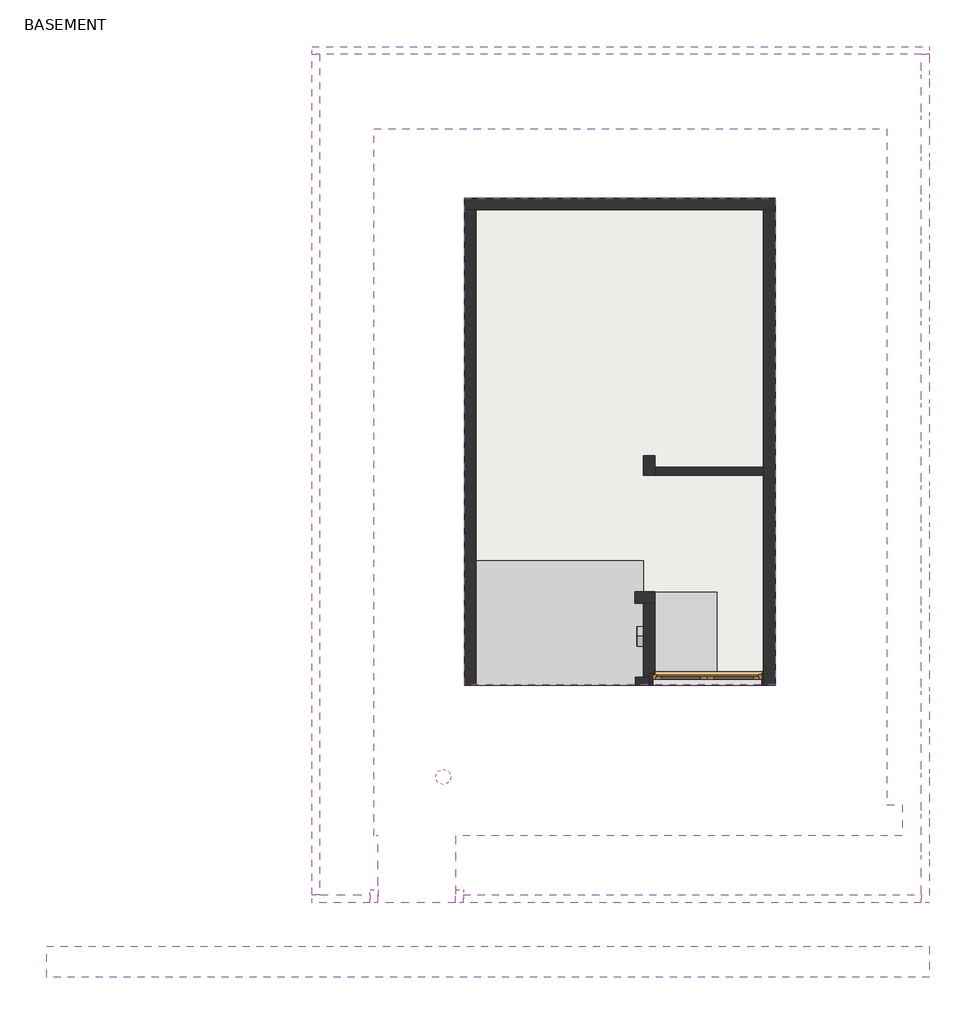
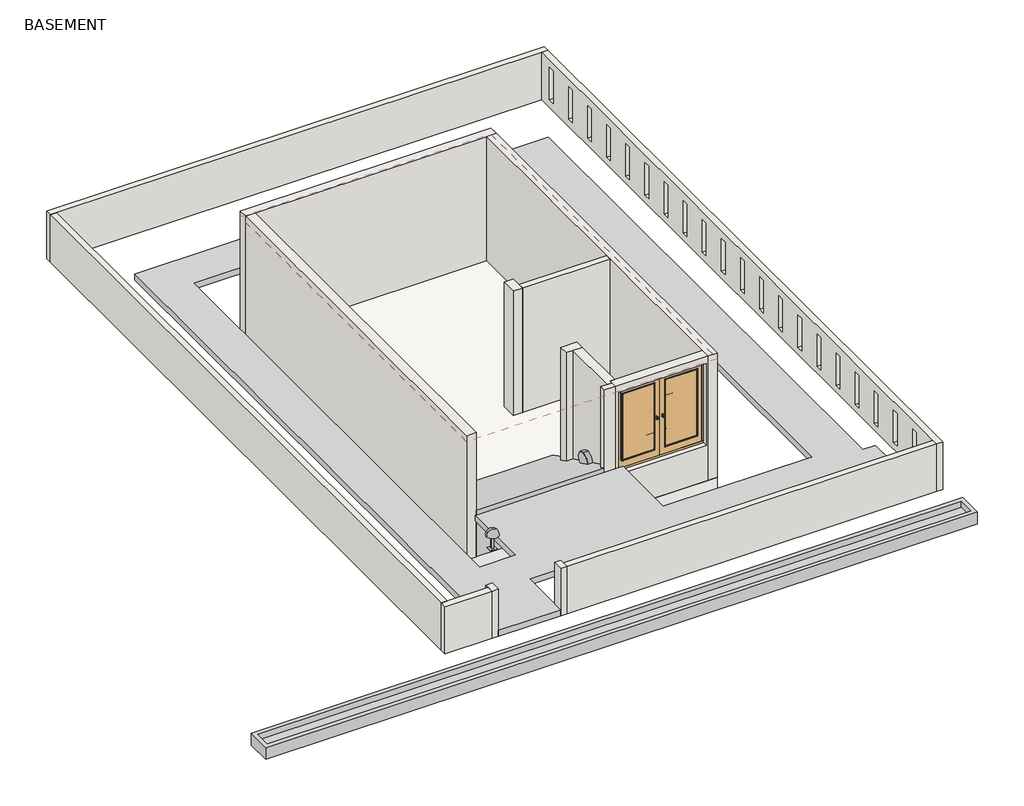
# One storey: 16 walls, 3 proxies, 2 light fixtures, 1 covering, 1 door, 1 slab.
"""IFC4 building model written with IfcOpenShell, lengths in millimetres."""

from ifc_helpers import new_model, si_unit, frame, origin, place, context, project, spatial, polyline, outline, extrude, faceted_brep, transform, mapped, element, save
from components import roads_a759df18, roads_ea5b5616, generic_models_1_generic_models_1_986dd2cf, extdbl_7_2134_x_2110mm_9b31339b, m_sconce_light_flat_round_60w_120v_dc625014, m_table_lamp_hemispheric_60w_120v_fef6e77c

model = new_model("IFC4")

# Units and contexts
model_context = context("Model", 3, world=origin())
ifc_project = project(units=[si_unit("LENGTHUNIT", "METRE", prefix="MILLI")], contexts=[model_context])

# Site, building, storey
site = spatial("IfcSite", under=ifc_project)
building = spatial("IfcBuilding", under=site)
storey = spatial("IfcBuildingStorey", under=building, Name="BASEMENT", Elevation=-3200.4)

# Proxies
placement = place(None, origin())
roads_shape = roads_a759df18(model_context)
element("IfcBuildingElementProxy", 1, Name="Roads", at=placement, inside=storey, context=model_context, shape_type="MappedRepresentation", body=[
    mapped(roads_shape, transform((0.0, 0.0, 0.0), x_axis=(1.0, 0.0, 0.0), y_axis=(0.0, 1.0, 0.0), z_axis=(0.0, 0.0, 1.0))),
])
roads_2_shape = roads_ea5b5616(model_context)
element("IfcBuildingElementProxy", 2, Name="Roads", at=placement, inside=storey, context=model_context, shape_type="MappedRepresentation", body=[
    mapped(roads_2_shape, transform((0.0, 0.0, 0.0), x_axis=(1.0, 0.0, 0.0), y_axis=(0.0, 1.0, 0.0), z_axis=(0.0, 0.0, 1.0))),
])
generic_models_1_generic_models_1_shape = generic_models_1_generic_models_1_986dd2cf(model_context)
element("IfcBuildingElementProxy", 3, Name="Generic Models 1 : Generic Models 1", ObjectType="Generic Models 1 : Generic Models 1", at=placement, inside=storey, context=model_context, shape_type="MappedRepresentation", body=[
    mapped(generic_models_1_generic_models_1_shape, transform((0.0, 0.0, 0.0), x_axis=(1.0, 0.0, 0.0), y_axis=(0.0, 1.0, 0.0), z_axis=(0.0, 0.0, 1.0))),
])

# Covering
element("IfcCovering", 4, ObjectType="2' x 4' ACT System", at=placement, inside=storey, context=model_context, shape_type="SweptSolid", body=[
    extrude(outline(polyline([(-23785.8963079, 6326.0742053), (-17689.8963079, 6326.0742053), (-17689.8963079, -3224.3257947), (-23785.8963079, -3224.3257947), (-23785.8963079, 6326.0742053)])), frame((0.0, 0.0, -152.4), z_axis=(0.0, 0.0, 1.0), x_axis=(1.0, 0.0, 0.0)), (0.0, 0.0, 1.0), 57.15),
])

# Door
extdbl_7_2134_x_2110mm_shape = extdbl_7_2134_x_2110mm_9b31339b(model_context)
element("IfcDoor", 5, ObjectType="ExtDbl (7) : 2134 x 2110mm", at=placement, inside=storey, context=model_context, shape_type="MappedRepresentation", body=[
    mapped(extdbl_7_2134_x_2110mm_shape, transform((-19022.2463079, -3110.0257947, -2286.0), x_axis=(1.0, 0.0, 0.0), y_axis=(0.0, 1.0, 0.0), z_axis=(0.0, 0.0, 1.0))),
])

# Light fixtures
m_sconce_light_flat_round_60w_120v_shape = m_sconce_light_flat_round_60w_120v_dc625014(model_context)
element("IfcLightFixture", 6, ObjectType="M_Sconce Light - Flat Round : 60W - 120V", at=placement, inside=storey, context=model_context, shape_type="MappedRepresentation", body=[
    mapped(m_sconce_light_flat_round_60w_120v_shape, transform((-20166.3963079, -2271.8257947, -4291.8211155), x_axis=(0.0, 1.0, 0.0), y_axis=(-1.0, 0.0, 0.0), z_axis=(0.0, 0.0, 1.0))),
])
m_table_lamp_hemispheric_60w_120v_shape = m_table_lamp_hemispheric_60w_120v_fef6e77c(model_context)
element("IfcLightFixture", 7, ObjectType="M_Table Lamp - Hemispheric : 60W - 120V", at=placement, inside=storey, context=model_context, shape_type="MappedRepresentation", body=[
    mapped(m_table_lamp_hemispheric_60w_120v_shape, transform((-24204.9963079, -5027.7257947, -1676.4), x_axis=(1.0, 0.0, 0.0), y_axis=(0.0, 1.0, 0.0), z_axis=(0.0, 0.0, 1.0))),
])

# Slab
element("IfcSlab", 8, ObjectType="Generic - 12\"", at=placement, inside=storey, context=model_context, shape_type="SweptSolid", body=[
    extrude(outline(polyline([(-23785.8963079, 6326.0742053), (-17689.8963079, 6326.0742053), (-17689.8963079, -3224.3257947), (-23785.8963079, -3224.3257947), (-23785.8963079, 6326.0742053)])), frame((0.0, 0.0, -3505.2), z_axis=(0.0, 0.0, 1.0), x_axis=(1.0, 0.0, 0.0)), (0.0, 0.0, 1.0), 304.8),
])

# Walls
element("IfcWall", 9, ObjectType="Generic - 6\"", at=placement, inside=storey, context=model_context, shape_type="SweptSolid", body=[
    extrude(outline(polyline([(-20052.0963079, 1042.8742053), (-17918.4963079, 1042.8742053), (-17918.4963079, 890.4742053), (-20052.0963079, 890.4742053), (-20052.0963079, 1042.8742053)])), frame((0.0, 0.0, -3200.4), z_axis=(0.0, 0.0, 1.0), x_axis=(1.0, 0.0, 0.0)), (0.0, 0.0, 1.0), 3200.4),
])
element("IfcWall", 10, ObjectType="Generic - 6\"", at=placement, inside=storey, context=model_context, shape_type="Brep", body=[
    faceted_brep([(-20433.0963079, -3224.3257947, -3200.4), (-20166.3963079, -3224.3257947, -3200.4), (-20166.3963079, -3224.3257947, 0.0), (-20433.0963079, -3224.3257947, 0.0), (-20433.0963079, -3071.9257947, -3200.4), (-20433.0963079, -3071.9257947, 0.0), (-20280.6963079, -3071.9257947, 0.0), (-20166.3963079, -3071.9257947, 0.0), (-20166.3963079, -3071.9257947, -3200.4), (-20280.6963079, -3071.9257947, -3200.4)], [[[0, 1, 2, 3]], [[4, 5, 6, 7, 8, 9]], [[1, 0, 4, 9, 8]], [[2, 1, 8, 7]], [[3, 2, 7, 6, 5]], [[0, 3, 5, 4]]]),
])
element("IfcWall", 11, ObjectType="Generic - 6\"", at=placement, inside=storey, context=model_context, shape_type="Brep", body=[
    faceted_brep([(-26783.0963079, 9145.4742053, -1981.2), (-26630.6963079, 9145.4742053, -1981.2), (-14819.6963079, 9145.4742053, -1981.2), (-14667.2963079, 9145.4742053, -1981.2), (-14667.2963079, 9145.4742053, -762.0), (-14819.6963079, 9145.4742053, -762.0), (-26630.6963079, 9145.4742053, -762.0), (-26783.0963079, 9145.4742053, -762.0), (-26783.0963079, 9297.8742053, -1981.2), (-26783.0963079, 9297.8742053, -762.0), (-14667.2963079, 9297.8742053, -762.0), (-14667.2963079, 9297.8742053, -1981.2)], [[[0, 1, 2, 3, 4, 5, 6, 7]], [[8, 9, 10, 11]], [[3, 2, 1, 0, 8, 11]], [[7, 6, 5, 4, 10, 9]], [[4, 3, 11, 10]], [[0, 7, 9, 8]]]),
])
element("IfcWall", 12, ObjectType="Generic - 6\"", at=placement, inside=storey, context=model_context, shape_type="Brep", body=[
    faceted_brep([(-14819.6963079, 9145.4742053, -1981.2), (-14819.6963079, -7339.1257947, -1981.2), (-14819.6963079, -7491.5257947, -1981.2), (-14819.6963079, -7491.5257947, -762.0), (-14819.6963079, -7339.1257947, -762.0), (-14819.6963079, 9145.4742053, -762.0), (-14819.6963079, -6490.3219748, -982.1857398), (-14819.6963079, -6642.4176399, -982.1857398), (-14819.6963079, -6642.4176399, -1818.7118977), (-14819.6963079, -6490.3219748, -1818.7118977), (-14819.6963079, 8667.8340702, -1794.1092134), (-14819.6963079, 8819.9297353, -1794.1092134), (-14819.6963079, 8819.9297353, -957.5830554), (-14819.6963079, 8667.8340702, -957.5830554), (-14819.6963079, 8014.1270137, -1795.4040915), (-14819.6963079, 8014.1270137, -958.8779336), (-14819.6963079, 7862.0313486, -958.8779336), (-14819.6963079, 7862.0313486, -1795.4040915), (-14819.6963079, 7208.3242921, -1796.6989696), (-14819.6963079, 7208.3242921, -960.1728117), (-14819.6963079, 7056.228627, -960.1728117), (-14819.6963079, 7056.228627, -1796.6989696), (-14819.6963079, 6402.5215705, -1797.9938477), (-14819.6963079, 6402.5215705, -961.4676898), (-14819.6963079, 6250.4259054, -961.4676898), (-14819.6963079, 6250.4259054, -1797.9938477), (-14819.6963079, 5596.7188489, -1799.2887259), (-14819.6963079, 5596.7188489, -962.7625679), (-14819.6963079, 5444.6231838, -962.7625679), (-14819.6963079, 5444.6231838, -1799.2887259), (-14819.6963079, 4790.9161273, -1800.583604), (-14819.6963079, 4790.9161273, -964.057446), (-14819.6963079, 4638.8204623, -964.057446), (-14819.6963079, 4638.8204623, -1800.583604), (-14819.6963079, 3985.1134058, -1801.8784821), (-14819.6963079, 3985.1134058, -965.3523242), (-14819.6963079, 3833.0177407, -965.3523242), (-14819.6963079, 3833.0177407, -1801.8784821), (-14819.6963079, 3179.3106842, -1803.1733602), (-14819.6963079, 3179.3106842, -966.6472023), (-14819.6963079, 3027.2150191, -966.6472023), (-14819.6963079, 3027.2150191, -1803.1733602), (-14819.6963079, 2373.5079626, -1804.4682384), (-14819.6963079, 2373.5079626, -967.9420804), (-14819.6963079, 2221.4122975, -967.9420804), (-14819.6963079, 2221.4122975, -1804.4682384), (-14819.6963079, 1567.705241, -1805.7631165), (-14819.6963079, 1567.705241, -969.2369585), (-14819.6963079, 1415.6095759, -969.2369585), (-14819.6963079, 1415.6095759, -1805.7631165), (-14819.6963079, 761.9025194, -1807.0579946), (-14819.6963079, 761.9025194, -970.5318367), (-14819.6963079, 609.8068543, -970.5318367), (-14819.6963079, 609.8068543, -1807.0579946), (-14819.6963079, -43.9002022, -1808.3528727), (-14819.6963079, -43.9002022, -971.8267148), (-14819.6963079, -195.9958672, -971.8267148), (-14819.6963079, -195.9958672, -1808.3528727), (-14819.6963079, -849.7029238, -1809.6477508), (-14819.6963079, -849.7029238, -973.1215929), (-14819.6963079, -1001.7985888, -973.1215929), (-14819.6963079, -1001.7985888, -1809.6477508), (-14819.6963079, -1655.5056453, -1810.942629), (-14819.6963079, -1655.5056453, -974.416471), (-14819.6963079, -1807.6013104, -974.416471), (-14819.6963079, -1807.6013104, -1810.942629), (-14819.6963079, -2461.3083669, -1812.2375071), (-14819.6963079, -2461.3083669, -975.7113492), (-14819.6963079, -2613.404032, -975.7113492), (-14819.6963079, -2613.404032, -1812.2375071), (-14819.6963079, -3267.1110885, -1813.5323852), (-14819.6963079, -3267.1110885, -977.0062273), (-14819.6963079, -3419.2067536, -977.0062273), (-14819.6963079, -3419.2067536, -1813.5323852), (-14819.6963079, -4072.9138101, -1814.8272633), (-14819.6963079, -4072.9138101, -978.3011054), (-14819.6963079, -4225.0094752, -978.3011054), (-14819.6963079, -4225.0094752, -1814.8272633), (-14819.6963079, -4878.7165317, -1816.1221415), (-14819.6963079, -4878.7165317, -979.5959835), (-14819.6963079, -5030.8121968, -979.5959835), (-14819.6963079, -5030.8121968, -1816.1221415), (-14819.6963079, -5684.5192533, -980.8908616), (-14819.6963079, -5836.6149183, -980.8908616), (-14819.6963079, -5836.6149183, -1817.4170196), (-14819.6963079, -5684.5192533, -1817.4170196), (-14667.2963079, -7491.5257947, -1981.2), (-14667.2963079, 9145.4742053, -1981.2), (-14667.2963079, 9145.4742053, -762.0), (-14667.2963079, -7491.5257947, -762.0), (-14667.2963079, -6642.4176399, -982.1857398), (-14667.2963079, -6490.3219748, -982.1857398), (-14667.2963079, -6490.3219748, -1818.7118977), (-14667.2963079, -6642.4176399, -1818.7118977), (-14667.2963079, 8819.9297353, -1794.1092134), (-14667.2963079, 8667.8340702, -1794.1092134), (-14667.2963079, 8667.8340702, -957.5830554), (-14667.2963079, 8819.9297353, -957.5830554), (-14667.2963079, 8014.1270137, -958.8779336), (-14667.2963079, 8014.1270137, -1795.4040915), (-14667.2963079, 7862.0313486, -1795.4040915), (-14667.2963079, 7862.0313486, -958.8779336), (-14667.2963079, 7208.3242921, -960.1728117), (-14667.2963079, 7208.3242921, -1796.6989696), (-14667.2963079, 7056.228627, -1796.6989696), (-14667.2963079, 7056.228627, -960.1728117), (-14667.2963079, 6402.5215705, -961.4676898), (-14667.2963079, 6402.5215705, -1797.9938477), (-14667.2963079, 6250.4259054, -1797.9938477), (-14667.2963079, 6250.4259054, -961.4676898), (-14667.2963079, 5596.7188489, -962.7625679), (-14667.2963079, 5596.7188489, -1799.2887259), (-14667.2963079, 5444.6231838, -1799.2887259), (-14667.2963079, 5444.6231838, -962.7625679), (-14667.2963079, 4790.9161273, -964.057446), (-14667.2963079, 4790.9161273, -1800.583604), (-14667.2963079, 4638.8204623, -1800.583604), (-14667.2963079, 4638.8204623, -964.057446), (-14667.2963079, 3985.1134058, -965.3523242), (-14667.2963079, 3985.1134058, -1801.8784821), (-14667.2963079, 3833.0177407, -1801.8784821), (-14667.2963079, 3833.0177407, -965.3523242), (-14667.2963079, 3179.3106842, -966.6472023), (-14667.2963079, 3179.3106842, -1803.1733602), (-14667.2963079, 3027.2150191, -1803.1733602), (-14667.2963079, 3027.2150191, -966.6472023), (-14667.2963079, 2373.5079626, -967.9420804), (-14667.2963079, 2373.5079626, -1804.4682384), (-14667.2963079, 2221.4122975, -1804.4682384), (-14667.2963079, 2221.4122975, -967.9420804), (-14667.2963079, 1567.705241, -969.2369585), (-14667.2963079, 1567.705241, -1805.7631165), (-14667.2963079, 1415.6095759, -1805.7631165), (-14667.2963079, 1415.6095759, -969.2369585), (-14667.2963079, 761.9025194, -970.5318367), (-14667.2963079, 761.9025194, -1807.0579946), (-14667.2963079, 609.8068543, -1807.0579946), (-14667.2963079, 609.8068543, -970.5318367), (-14667.2963079, -43.9002022, -971.8267148), (-14667.2963079, -43.9002022, -1808.3528727), (-14667.2963079, -195.9958672, -1808.3528727), (-14667.2963079, -195.9958672, -971.8267148), (-14667.2963079, -849.7029238, -973.1215929), (-14667.2963079, -849.7029238, -1809.6477508), (-14667.2963079, -1001.7985888, -1809.6477508), (-14667.2963079, -1001.7985888, -973.1215929), (-14667.2963079, -1655.5056453, -974.416471), (-14667.2963079, -1655.5056453, -1810.942629), (-14667.2963079, -1807.6013104, -1810.942629), (-14667.2963079, -1807.6013104, -974.416471), (-14667.2963079, -2461.3083669, -975.7113492), (-14667.2963079, -2461.3083669, -1812.2375071), (-14667.2963079, -2613.404032, -1812.2375071), (-14667.2963079, -2613.404032, -975.7113492), (-14667.2963079, -3267.1110885, -977.0062273), (-14667.2963079, -3267.1110885, -1813.5323852), (-14667.2963079, -3419.2067536, -1813.5323852), (-14667.2963079, -3419.2067536, -977.0062273), (-14667.2963079, -4072.9138101, -978.3011054), (-14667.2963079, -4072.9138101, -1814.8272633), (-14667.2963079, -4225.0094752, -1814.8272633), (-14667.2963079, -4225.0094752, -978.3011054), (-14667.2963079, -4878.7165317, -979.5959835), (-14667.2963079, -4878.7165317, -1816.1221415), (-14667.2963079, -5030.8121968, -1816.1221415), (-14667.2963079, -5030.8121968, -979.5959835), (-14667.2963079, -5836.6149183, -980.8908616), (-14667.2963079, -5684.5192533, -980.8908616), (-14667.2963079, -5684.5192533, -1817.4170196), (-14667.2963079, -5836.6149183, -1817.4170196)], [[[0, 1, 2, 3, 4, 5], [6, 7, 8, 9], [10, 11, 12, 13], [14, 15, 16, 17], [18, 19, 20, 21], [22, 23, 24, 25], [26, 27, 28, 29], [30, 31, 32, 33], [34, 35, 36, 37], [38, 39, 40, 41], [42, 43, 44, 45], [46, 47, 48, 49], [50, 51, 52, 53], [54, 55, 56, 57], [58, 59, 60, 61], [62, 63, 64, 65], [66, 67, 68, 69], [70, 71, 72, 73], [74, 75, 76, 77], [78, 79, 80, 81], [82, 83, 84, 85]], [[86, 87, 88, 89], [90, 91, 92, 93], [94, 95, 96, 97], [98, 99, 100, 101], [102, 103, 104, 105], [106, 107, 108, 109], [110, 111, 112, 113], [114, 115, 116, 117], [118, 119, 120, 121], [122, 123, 124, 125], [126, 127, 128, 129], [130, 131, 132, 133], [134, 135, 136, 137], [138, 139, 140, 141], [142, 143, 144, 145], [146, 147, 148, 149], [150, 151, 152, 153], [154, 155, 156, 157], [158, 159, 160, 161], [162, 163, 164, 165], [166, 167, 168, 169]], [[2, 1, 0, 87, 86]], [[5, 4, 3, 89, 88]], [[0, 5, 88, 87]], [[3, 2, 86, 89]], [[6, 91, 90, 7]], [[8, 93, 92, 9]], [[91, 6, 9, 92]], [[7, 90, 93, 8]], [[12, 97, 96, 13]], [[10, 95, 94, 11]], [[97, 12, 11, 94]], [[13, 96, 95, 10]], [[15, 98, 101, 16]], [[17, 100, 99, 14]], [[98, 15, 14, 99]], [[16, 101, 100, 17]], [[19, 102, 105, 20]], [[21, 104, 103, 18]], [[102, 19, 18, 103]], [[20, 105, 104, 21]], [[23, 106, 109, 24]], [[25, 108, 107, 22]], [[106, 23, 22, 107]], [[24, 109, 108, 25]], [[27, 110, 113, 28]], [[29, 112, 111, 26]], [[110, 27, 26, 111]], [[28, 113, 112, 29]], [[31, 114, 117, 32]], [[33, 116, 115, 30]], [[114, 31, 30, 115]], [[32, 117, 116, 33]], [[35, 118, 121, 36]], [[37, 120, 119, 34]], [[118, 35, 34, 119]], [[36, 121, 120, 37]], [[39, 122, 125, 40]], [[41, 124, 123, 38]], [[122, 39, 38, 123]], [[40, 125, 124, 41]], [[43, 126, 129, 44]], [[45, 128, 127, 42]], [[126, 43, 42, 127]], [[44, 129, 128, 45]], [[47, 130, 133, 48]], [[49, 132, 131, 46]], [[130, 47, 46, 131]], [[48, 133, 132, 49]], [[51, 134, 137, 52]], [[53, 136, 135, 50]], [[134, 51, 50, 135]], [[52, 137, 136, 53]], [[55, 138, 141, 56]], [[57, 140, 139, 54]], [[138, 55, 54, 139]], [[56, 141, 140, 57]], [[59, 142, 145, 60]], [[61, 144, 143, 58]], [[142, 59, 58, 143]], [[60, 145, 144, 61]], [[63, 146, 149, 64]], [[65, 148, 147, 62]], [[146, 63, 62, 147]], [[64, 149, 148, 65]], [[67, 150, 153, 68]], [[69, 152, 151, 66]], [[150, 67, 66, 151]], [[68, 153, 152, 69]], [[71, 154, 157, 72]], [[73, 156, 155, 70]], [[154, 71, 70, 155]], [[72, 157, 156, 73]], [[75, 158, 161, 76]], [[77, 160, 159, 74]], [[158, 75, 74, 159]], [[76, 161, 160, 77]], [[79, 162, 165, 80]], [[81, 164, 163, 78]], [[162, 79, 78, 163]], [[80, 165, 164, 81]], [[82, 167, 166, 83]], [[84, 169, 168, 85]], [[167, 82, 85, 168]], [[83, 166, 169, 84]]]),
])
element("IfcWall", 13, ObjectType="Generic - 6\"", at=placement, inside=storey, context=model_context, shape_type="SweptSolid", body=[
    extrude(outline(polyline([(-23811.2963079, -7339.1257947), (-14819.6963079, -7339.1257947), (-14819.6963079, -7491.5257947), (-23811.2963079, -7491.5257947), (-23811.2963079, -7339.1257947)])), frame((0.0, 0.0, -1981.2), z_axis=(0.0, 0.0, 1.0), x_axis=(1.0, 0.0, 0.0)), (0.0, 0.0, 1.0), 1219.2),
])
element("IfcWall", 14, ObjectType="Generic - 6\"", at=placement, inside=storey, context=model_context, shape_type="SweptSolid", body=[
    extrude(outline(polyline([(-26630.6963079, 9145.4742053), (-26630.6963079, -7339.1257947), (-26783.0963079, -7339.1257947), (-26783.0963079, 9145.4742053), (-26630.6963079, 9145.4742053)])), frame((0.0, 0.0, -1981.2), z_axis=(0.0, 0.0, 1.0), x_axis=(1.0, 0.0, 0.0)), (0.0, 0.0, 1.0), 1219.2),
])
element("IfcWall", 15, ObjectType="Generic - 6\"", at=placement, inside=storey, context=model_context, shape_type="Brep", body=[
    faceted_brep([(-25640.0963079, -7339.1257947, -1981.2), (-26630.6963079, -7339.1257947, -1981.2), (-26783.0963079, -7339.1257947, -1981.2), (-26783.0963079, -7339.1257947, -762.0), (-26630.6963079, -7339.1257947, -762.0), (-25640.0963079, -7339.1257947, -762.0), (-25640.0963079, -7491.5257947, -1981.2), (-25640.0963079, -7491.5257947, -762.0), (-26783.0963079, -7491.5257947, -762.0), (-26783.0963079, -7491.5257947, -1981.2)], [[[0, 1, 2, 3, 4, 5]], [[6, 7, 8, 9]], [[2, 1, 0, 6, 9]], [[5, 4, 3, 8, 7]], [[3, 2, 9, 8]], [[0, 5, 7, 6]]]),
])
element("IfcWall", 16, ObjectType="Generic - 6\"", at=placement, inside=storey, context=model_context, shape_type="Brep", body=[
    faceted_brep([(-25487.6963079, -7491.5257947, -1981.2), (-25487.6963079, -7237.5257947, -1981.2), (-25487.6963079, -7237.5257947, -762.0), (-25487.6963079, -7491.5257947, -762.0), (-25640.0963079, -7491.5257947, -1981.2), (-25640.0963079, -7491.5257947, -762.0), (-25640.0963079, -7339.1257947, -762.0), (-25640.0963079, -7237.5257947, -762.0), (-25640.0963079, -7237.5257947, -1981.2), (-25640.0963079, -7339.1257947, -1981.2)], [[[0, 1, 2, 3]], [[4, 5, 6, 7, 8, 9]], [[1, 0, 4, 9, 8]], [[2, 1, 8, 7]], [[3, 2, 7, 6, 5]], [[0, 3, 5, 4]]]),
])
element("IfcWall", 17, ObjectType="Generic - 6\"", at=placement, inside=storey, context=model_context, shape_type="Brep", body=[
    faceted_brep([(-23811.2963079, -7491.5257947, -1981.2), (-23811.2963079, -7339.1257947, -1981.2), (-23811.2963079, -7237.5257947, -1981.2), (-23811.2963079, -7237.5257947, -762.0), (-23811.2963079, -7339.1257947, -762.0), (-23811.2963079, -7491.5257947, -762.0), (-23963.6963079, -7491.5257947, -1981.2), (-23963.6963079, -7491.5257947, -762.0), (-23963.6963079, -7237.5257947, -762.0), (-23963.6963079, -7237.5257947, -1981.2)], [[[0, 1, 2, 3, 4, 5]], [[6, 7, 8, 9]], [[2, 1, 0, 6, 9]], [[3, 2, 9, 8]], [[5, 4, 3, 8, 7]], [[0, 5, 7, 6]]]),
])
element("IfcWall", 18, ObjectType="Generic - 9\"", at=placement, inside=storey, context=model_context, shape_type="Brep", body=[
    faceted_brep([(-23785.8963079, 6097.4742053, -3200.4), (-23557.2963079, 6097.4742053, -3200.4), (-17918.4963079, 6097.4742053, -3200.4), (-17689.8963079, 6097.4742053, -3200.4), (-17689.8963079, 6097.4742053, 0.0), (-17918.4963079, 6097.4742053, 0.0), (-23557.2963079, 6097.4742053, 0.0), (-23785.8963079, 6097.4742053, 0.0), (-23785.8963079, 6326.0742053, -3200.4), (-23785.8963079, 6326.0742053, 0.0), (-17689.8963079, 6326.0742053, 0.0), (-17689.8963079, 6326.0742053, -3200.4)], [[[0, 1, 2, 3, 4, 5, 6, 7]], [[8, 9, 10, 11]], [[3, 2, 1, 0, 8, 11]], [[7, 6, 5, 4, 10, 9]], [[0, 7, 9, 8]], [[4, 3, 11, 10]]]),
])
element("IfcWall", 19, ObjectType="Generic - 9\"", at=placement, inside=storey, context=model_context, shape_type="SweptSolid", body=[
    extrude(outline(polyline([(-23785.8963079, -3224.3257947), (-23785.8963079, 6097.4742053), (-23557.2963079, 6097.4742053), (-23557.2963079, -3224.3257947), (-23785.8963079, -3224.3257947)])), frame((0.0, 0.0, -3200.4), z_axis=(0.0, 0.0, 1.0), x_axis=(1.0, 0.0, 0.0)), (0.0, 0.0, 1.0), 3200.4),
])
element("IfcWall", 20, ObjectType="Generic - 9\"", at=placement, inside=storey, context=model_context, shape_type="Brep", body=[
    faceted_brep([(-17918.4963079, 6097.4742053, -3200.4), (-17918.4963079, 1042.8742053, -3200.4), (-17918.4963079, 890.4742053, -3200.4), (-17918.4963079, -2995.7257947, -3200.4), (-17918.4963079, -3224.3257947, -3200.4), (-17918.4963079, -3224.3257947, 0.0), (-17918.4963079, -2995.7257947, 0.0), (-17918.4963079, 890.4742053, 0.0), (-17918.4963079, 1042.8742053, 0.0), (-17918.4963079, 6097.4742053, 0.0), (-17689.8963079, 6097.4742053, -3200.4), (-17689.8963079, 6097.4742053, 0.0), (-17689.8963079, -3224.3257947, 0.0), (-17689.8963079, -3224.3257947, -3200.4)], [[[0, 1, 2, 3, 4, 5, 6, 7, 8, 9]], [[10, 11, 12, 13]], [[4, 3, 2, 1, 0, 10, 13]], [[9, 8, 7, 6, 5, 12, 11]], [[0, 9, 11, 10]], [[5, 4, 13, 12]]]),
])
element("IfcWall", 21, ObjectType="Generic - 9\"", at=placement, inside=storey, context=model_context, shape_type="Brep", body=[
    faceted_brep([(-17918.4963079, -2995.7257947, -3200.4), (-20052.0963079, -2995.7257947, -3200.4), (-20166.3963079, -2995.7257947, -3200.4), (-20166.3963079, -2995.7257947, 0.0), (-20052.0963079, -2995.7257947, 0.0), (-17918.4963079, -2995.7257947, 0.0), (-20089.0463079, -2995.7257947, -2286.0), (-17955.4463079, -2995.7257947, -2286.0), (-17955.4463079, -2995.7257947, -176.0), (-20089.0463079, -2995.7257947, -176.0), (-20166.3963079, -3224.3257947, -3200.4), (-17918.4963079, -3224.3257947, -3200.4), (-17918.4963079, -3224.3257947, 0.0), (-20166.3963079, -3224.3257947, 0.0), (-17955.4463079, -3224.3257947, -2286.0), (-20089.0463079, -3224.3257947, -2286.0), (-20089.0463079, -3224.3257947, -176.0), (-17955.4463079, -3224.3257947, -176.0), (-20166.3963079, -3071.9257947, -3200.4), (-20166.3963079, -3071.9257947, 0.0)], [[[0, 1, 2, 3, 4, 5], [6, 7, 8, 9]], [[10, 11, 12, 13], [14, 15, 16, 17]], [[2, 1, 0, 11, 10, 18]], [[3, 2, 18, 10, 13, 19]], [[5, 4, 3, 19, 13, 12]], [[0, 5, 12, 11]], [[6, 15, 14, 7]], [[7, 14, 17, 8]], [[8, 17, 16, 9]], [[15, 6, 9, 16]]]),
])
element("IfcWall", 22, ObjectType="Generic - 9\"", at=placement, inside=storey, context=model_context, shape_type="Brep", body=[
    faceted_brep([(-20280.6963079, 1271.4742053, -3200.4), (-20280.6963079, 890.4742053, -3200.4), (-20280.6963079, 890.4742053, 0.0), (-20280.6963079, 1271.4742053, 0.0), (-20052.0963079, 1271.4742053, -3200.4), (-20052.0963079, 1271.4742053, 0.0), (-20052.0963079, 1042.8742053, 0.0), (-20052.0963079, 890.4742053, 0.0), (-20052.0963079, 890.4742053, -3200.4), (-20052.0963079, 1042.8742053, -3200.4)], [[[0, 1, 2, 3]], [[4, 5, 6, 7, 8, 9]], [[1, 0, 4, 9, 8]], [[3, 2, 7, 6, 5]], [[0, 3, 5, 4]], [[2, 1, 8, 7]]]),
])
element("IfcWall", 23, ObjectType="Generic - 9\"", at=placement, inside=storey, context=model_context, shape_type="Brep", body=[
    faceted_brep([(-20280.6963079, -1624.1257947, -3200.4), (-20280.6963079, -3071.9257947, -3200.4), (-20280.6963079, -3071.9257947, 0.0), (-20280.6963079, -1624.1257947, 0.0), (-20052.0963079, -2995.7257947, -3200.4), (-20052.0963079, -1624.1257947, -3200.4), (-20052.0963079, -1624.1257947, 0.0), (-20052.0963079, -2995.7257947, 0.0), (-20052.0963079, -2995.7257947, -176.0), (-20052.0963079, -2995.7257947, -2286.0), (-20166.3963079, -2995.7257947, -3200.4), (-20166.3963079, -3071.9257947, -3200.4), (-20166.3963079, -3071.9257947, 0.0), (-20166.3963079, -2995.7257947, 0.0)], [[[0, 1, 2, 3]], [[4, 5, 6, 7, 8, 9]], [[1, 0, 5, 4, 10, 11]], [[3, 2, 12, 13, 7, 6]], [[2, 1, 11, 12]], [[11, 10, 13, 12]], [[10, 4, 9, 8, 7, 13]], [[0, 3, 6, 5]]]),
])
element("IfcWall", 24, ObjectType="Generic - 9\"", at=placement, inside=storey, context=model_context, shape_type="Brep", body=[
    faceted_brep([(-20445.7963079, -1624.1257947, -3200.4), (-20280.6963079, -1624.1257947, -3200.4), (-20052.0963079, -1624.1257947, -3200.4), (-20052.0963079, -1624.1257947, 0.0), (-20280.6963079, -1624.1257947, 0.0), (-20445.7963079, -1624.1257947, 0.0), (-20445.7963079, -1395.5257947, -3200.4), (-20445.7963079, -1395.5257947, 0.0), (-20052.0963079, -1395.5257947, 0.0), (-20052.0963079, -1395.5257947, -3200.4)], [[[0, 1, 2, 3, 4, 5]], [[6, 7, 8, 9]], [[2, 1, 0, 6, 9]], [[5, 4, 3, 8, 7]], [[0, 5, 7, 6]], [[3, 2, 9, 8]]]),
])

save(model, "model.ifc")

# Revit data of these elements
# Type "2' x 4' ACT System"
#   Assembly Code = "C3030210"
#   built-in parameter 1002203 = 1 (stored number, unit not read)
#   built-in parameter 1002202 = 1 (stored number, unit not read)
#   Layers, outside or top first: 0' - 1 5/8" "Default" (function 1); 0' - 0 5/8" "Acoustic Ceiling Tile 24 x 48" (function 5)
# Type "ExtDbl (7) : 2134 x 2110mm"
#   Type Mark = "15"
#   Operation = "DoubleDoorSingleSwing"
#   Keynote = "L20"
#   Wrap Layers (Ext) from Ext = 0' - 4.03543"
#   Wrap Layers (Int) from Ext = 0' - 6.98819"
#   Thickness = 0' - 1.73228"
#   Stile Top Rail = 0' - 3.93701"
#   Stile Shutting = 0' - 4.92126"
#   Stile Hanging = 0' - 3.93701"
#   Stile Bottom Rail = 0' - 6.88976"
#   Rough Width = 7' - 0"
#   Rough Height = 6' - 11.07087"
#   O/A Frame Width = 0' - 2.51969"
#   Handle Z Distance = 3' - 5.33858"
#   Glazing Thickness = 0' - 0.94488"
#   Glazing Bar Thickness = 0' - 0.7874"
#   Glazing Bar Inset = 0' - 2.95276"
#   FrameWidth = 0' - 1.65354"
#   FrameOffset - External = 0' - 0.98425"
#   FrameDepth = 0' - 3.50394"
#   Door Panel Width = 3' - 3.91339"
#   Door Panel Thickness = 0' - 1.73228"
#   Door Panel Height = 6' - 6.74016"
#   Cill Thickness = 0' - 2.14567"
#   Cill Projection = 0' - 1.1811"
#   Handle X Distance = 0' - 2.95276"
#   Height = 6' - 11.07087"
#   Structural Tolerance = 0' - 0.25591"
#   Tolerance = 0' - 0.11811"
#   Undercut = 0' - 0.15748"
#   Width = 7' - 0"
#   Cill Extension = 0' - 0.98425"
#   Cavity Closer Width = 0' - 1.9685"
#   Cavity Closer Offset from Ext = 0' - 4.03543"
#   Cavity Closer Depth = 0' - 3.34646"
#   Vis - Ironmongery = yes
#   Vis - Glazing Bars = yes
#   Vis - Cavity Closers = yes
#   Function = 1
#   Material Glass = Door - Glazing
#   Material Door = Door - Panel
#   Material Ironmongery = Door - Handle
#   Wall Closure = (empty or 0)
# Type "M_Sconce Light - Flat Round : 60W - 120V"
#   Assembly Code = "D5020220"
#   Lamp = "A-19"
#   Wattage = 60 W
#   built-in parameter 1150110 = 1 (stored number, unit not read)
#   built-in parameter 1114217 = 1 (stored number, unit not read)
#   built-in parameter 1150109 = 1 (stored number, unit not read)
#   built-in parameter 1150113 = 1 (stored number, unit not read)
#   built-in parameter 1150115 = 1 (stored number, unit not read)
#   built-in parameter 1150105 = 272.155 (stored number, unit not read)
#   Light Source Symbol Size = 2' - 0"
#   built-in parameter 1150112 = 1 (stored number, unit not read)
#   built-in parameter 1150114 = 1 (stored number, unit not read)
#   built-in parameter 1150107 = 2800 (stored number, unit not read)
#   built-in parameter 1150106 = 2.72155 (stored number, unit not read)
#   built-in parameter 1150104 = 1.32387 (stored number, unit not read)
#   Ballast Voltage = 120 V
#   built-in parameter 1114218 = 1 (stored number, unit not read)
#   built-in parameter 1150133 = 10 (stored number, unit not read)
#   Lumens = 855 lm
#   Mounting Height = 6' - 2.80315"
#   Radius = 0' - 7.87402"
#   Apparent Load = 60 VA
#   built-in parameter 1150134 = 4
#   built-in parameter 1150137 = 1
#   Color Filter = 16777215
#   built-in parameter 1140040 [instance default] = 1
#   Ballast Number of Poles = 1
#   Shade Material = Glass, Frosted
#   Dimming Lamp Color Temperature Shift = (empty or 0)
#   Default Elevation = 0
#   Wattage Comments = ""
# Type "M_Table Lamp - Hemispheric : 60W - 120V"
#   Photometric Web File = "TLAE1A19.ies"
#   Assembly Code = "D5020220"
#   Lamp = "A-19"
#   Wattage = 60 W
#   built-in parameter 1150110 = 1 (stored number, unit not read)
#   built-in parameter 1114217 = 1 (stored number, unit not read)
#   built-in parameter 1150109 = 1 (stored number, unit not read)
#   built-in parameter 1150113 = 1 (stored number, unit not read)
#   Tilt Angle = 90.00°
#   built-in parameter 1150115 = 1 (stored number, unit not read)
#   built-in parameter 1150105 = 68.0387 (stored number, unit not read)
#   built-in parameter 1150112 = 1 (stored number, unit not read)
#   built-in parameter 1150114 = 1 (stored number, unit not read)
#   built-in parameter 1150107 = 2800 (stored number, unit not read)
#   built-in parameter 1150106 = 0.680387 (stored number, unit not read)
#   built-in parameter 1150104 = 1.32387 (stored number, unit not read)
#   Voltage = 120 V
#   built-in parameter 1114218 = 1 (stored number, unit not read)
#   built-in parameter 1150133 = 10 (stored number, unit not read)
#   Lumens = 855 lm
#   Apparent Load = 60 VA
#   built-in parameter 1150134 = 4
#   built-in parameter 1150137 = 1
#   Color Filter = 16777215
#   Number of poles = 1
#   Mount Material = Steel, Chrome Plated
#   Shade Material = Plastic, Lamp Shade
#   Base Material = Birch
#   Dimming Lamp Color Temperature Shift = (empty or 0)
#   Default Elevation = 0
#   Wattage Comments = ""
# Type "Generic - 12\""
#   Assembly Code = "B1010"
#   Function = 0
#   Layers, outside or top first: 1' - 0" no material (function 1)
# Type "Generic - 6\""
#   Assembly Code = "B2010"
#   Layers, outside or top first: 0' - 6" no material (function 1)
# Type "Generic - 9\""
#   Assembly Code = "B2010"
#   Layers, outside or top first: 0' - 9" no material (function 1)
# Element 1 (IfcBuildingElementProxy)
#   Phase Created = New Construction
#   Materials on its faces: "Damp-proofing"
# Element 2 (IfcBuildingElementProxy)
#   Phase Created = New Construction
# Element 3 (IfcBuildingElementProxy, "Generic Models 1 : Generic Models 1")
#   Phase Created = New Construction
# Element 4 (IfcCovering, "2' x 4' ACT System")
#   Height Offset From Level = 10' - 0"
#   Phase Created = New Construction
#   Materials on its faces: "Acoustic Ceiling Tile 24 x 48", "Default"
# Element 5 (IfcDoor, "ExtDbl (7) : 2134 x 2110mm")
#   Phase Created = New Construction
#   Materials on its faces: "Door - Panel", "Door - Handle", "Door - Glazing"
# Element 6 (IfcLightFixture, "M_Sconce Light - Flat Round : 60W - 120V")
#   Mark = "15"
#   built-in parameter 1140040 = 1
#   Phase Created = New Construction
#   Materials on its faces: "Glass, Frosted"
# Element 7 (IfcLightFixture, "M_Table Lamp - Hemispheric : 60W - 120V")
#   Mark = "12"
#   Phase Created = New Construction
#   Materials on its faces: "Steel, Chrome Plated", "Birch", "Plastic, Lamp Shade"
# Element 8 (IfcSlab, "Generic - 12\"")
#   built-in parameter 1001955 = 1.5708 (stored number, unit not read)
#   Height Offset From Level = 0' - 0"
#   Phase Created = New Construction
#   Materials on its faces: "Default Floor", "Concrete, Cast-in-Place gray"
# Element 9 (IfcWall, "Generic - 6\"")
#   Top Offset = 0' - 0"
#   Base Offset = 0' - 0"
#   Unconnected Height = 10' - 6"
#   wall height = 10' - 6"
#   Phase Created = New Construction
#   Base Constraint = BASEMENT
#   Materials on its faces: "Default Wall"
# Element 10 (IfcWall, "Generic - 6\"")
#   Top Offset = 0' - 0"
#   Base Offset = 0' - 0"
#   Unconnected Height = 10' - 6"
#   wall height = 10' - 6"
#   Phase Created = New Construction
#   Base Constraint = BASEMENT
#   Materials on its faces: "Default Wall", "Parking Stripe"
# Elements 11, 13 (IfcWall, "Generic - 6\"")
#   built-in parameter 1001111 = 4' - 0"
#   Top Offset = 0' - 0"
#   Base Offset = 4' - 0"
#   Unconnected Height = 4' - 0"
#   wall height = 4' - 0"
#   Phase Created = New Construction
#   Base Constraint = BASEMENT
#   Materials on its faces: "3D plant-4", "Default Wall"
# Elements 12, 14 (IfcWall, "Generic - 6\"")
#   built-in parameter 1001111 = 4' - 0"
#   Top Offset = 0' - 0"
#   Base Offset = 4' - 0"
#   Unconnected Height = 4' - 0"
#   wall height = 4' - 0"
#   Phase Created = New Construction
#   Base Constraint = BASEMENT
#   Materials on its faces: "Default Wall", "3D plant-4"
# Elements 15, 17 (IfcWall, "Generic - 6\"")
#   built-in parameter 1001111 = 4' - 0"
#   Top Offset = 0' - 0"
#   Base Offset = 4' - 0"
#   Unconnected Height = 4' - 0"
#   wall height = 4' - 0"
#   Phase Created = New Construction
#   Base Constraint = BASEMENT
#   Materials on its faces: "Default Wall", "Parking Stripe", "3D plant-4"
# Element 16 (IfcWall, "Generic - 6\"")
#   built-in parameter 1001111 = 4' - 0"
#   Top Offset = 0' - 0"
#   Base Offset = 4' - 0"
#   Unconnected Height = 4' - 0"
#   wall height = 4' - 0"
#   Phase Created = New Construction
#   Base Constraint = BASEMENT
#   Materials on its faces: "Parking Stripe", "Default Wall"
# Elements 18, 19, 20, 23, 24 (IfcWall, "Generic - 9\"")
#   Top Offset = 0' - 0"
#   Base Offset = 0' - 0"
#   Unconnected Height = 10' - 6"
#   wall height = 10' - 6"
#   Phase Created = New Construction
#   Base Constraint = BASEMENT
#   Materials on its faces: "Default Wall", "Parking Stripe"
# Elements 21, 22 (IfcWall, "Generic - 9\"")
#   Top Offset = 0' - 0"
#   Base Offset = 0' - 0"
#   Unconnected Height = 10' - 6"
#   wall height = 10' - 6"
#   Phase Created = New Construction
#   Base Constraint = BASEMENT
#   Materials on its faces: "Default Wall"
# Materials
#   "Default": colour RGB 80 80 80, transparency 0
#   "Acoustic Ceiling Tile 24 x 48": class "Generic", colour RGB 180 179 177, transparency 0, Description = "Acoustic Ceiling Tile 24 x 48", Cost = 0
#   "Door - Glazing": colour RGB 0 0 255, transparency 0.75
#   "Door - Panel": class "Wood", colour RGB 114 82 51, transparency 0
#   "Door - Handle": colour RGB 247 247 247, transparency 0
#   "Glass, Frosted": class "Glass", colour RGB 250 244 225, transparency 0.55, Description = "physical material", Cost = 0
#   "Steel, Chrome Plated": class "Metal", colour RGB 244 244 244, transparency 0, Description = "Chromiuim plated steel", Cost = 0
#   "Plastic, Lamp Shade": class "Glass", colour RGB 250 244 225, transparency 0.58, Description = "physical material", Cost = 0
#   "Birch": class "Wood", colour RGB 224 178 126, transparency 0, Description = "Betula Alleghaniensis", Cost = 0
#   "Damp-proofing": class "Generic", colour RGB 17 17 17, transparency 0, Description = "Damp-proofing", Cost = 0
#   "Default Floor": colour RGB 80 80 80, transparency 0
#   "Concrete, Cast-in-Place gray": class "Concrete", colour RGB 115 116 108, transparency 0, Description = "Cast-in-place concrete", Cost = 0
#   "Default Wall": colour RGB 80 80 80, transparency 0
#   "Parking Stripe": class "Paint", colour RGB 226 219 42, transparency 0
#   "3D plant-4": class "Paint", colour RGB 165 165 82, transparency 0
